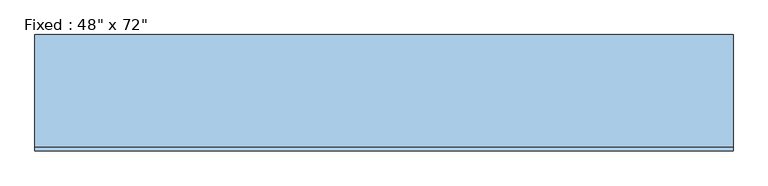
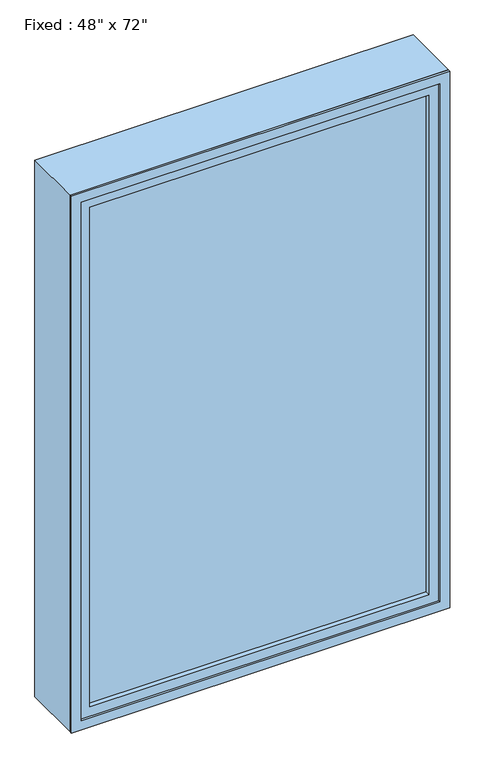
"""IFC4 building model written with IfcOpenShell, lengths in millimetres: window geometry."""

from ifc_helpers import new_model, si_unit, frame, origin, place, context, project, spatial, polyline, outline, extrude, source, transform, mapped, element, save


def window_b4876e44(model_context):
    return source(origin(), model_context, "Body", "SweptSolid", [
        extrude(outline(polyline([(508.0, -79.375), (-584.2, -79.375), (-584.2, -66.675), (508.0, -66.675), (508.0, -79.375)])), frame((0.0, 0.0, 368.3), z_axis=(0.0, 0.0, 1.0), x_axis=(1.0, 0.0, 0.0)), (0.0, 0.0, 1.0), 1701.8),
        extrude(outline(polyline([(2114.55, -628.65), (323.85, -628.65), (323.85, 552.45), (2114.55, 552.45), (2114.55, -628.65)]), holes=[polyline([(2070.1, -584.2), (2070.1, 508.0), (368.3, 508.0), (368.3, -584.2), (2070.1, -584.2)])]), frame((0.0, -95.25, 0.0), z_axis=(0.0, 1.0, 0.0), x_axis=(0.0, 0.0, 1.0)), (0.0, 0.0, 1.0), 44.45),
        extrude(outline(polyline([(2133.6, -647.7), (304.8, -647.7), (304.8, 571.5), (2133.6, 571.5), (2133.6, -647.7)]), holes=[polyline([(2101.85, -615.95), (2101.85, 539.75), (336.55, 539.75), (336.55, -615.95), (2101.85, -615.95)])]), frame((0.0, -101.6, 0.0), z_axis=(0.0, 1.0, 0.0), x_axis=(0.0, 0.0, 1.0)), (0.0, 0.0, 1.0), 6.35),
        extrude(outline(polyline([(2133.6, 571.5), (2133.6, -647.7), (304.8, -647.7), (304.8, 571.5), (2133.6, 571.5)]), holes=[polyline([(2114.55, 552.45), (323.85, 552.45), (323.85, -628.65), (2114.55, -628.65), (2114.55, 552.45)])]), frame((0.0, -95.25, 0.0), z_axis=(0.0, 1.0, 0.0), x_axis=(0.0, 0.0, 1.0)), (0.0, 0.0, 1.0), 196.85),
    ])


if __name__ == "__main__":
    model = new_model("IFC4")
    model_context = context("Model", 3, world=origin())
    ifc_project = project(units=[si_unit("LENGTHUNIT", "METRE", prefix="MILLI")], contexts=[model_context])
    site = spatial("IfcSite", under=ifc_project)
    building = spatial("IfcBuilding", under=site)
    placement = place(None, origin())
    window_shape = window_b4876e44(model_context)
    element("IfcWindow", 1, ObjectType="Fixed : 48\" x 72\"", at=placement, inside=building, context=model_context, shape_type="MappedRepresentation", body=[
        mapped(window_shape, transform((0.0, 0.0, 0.0), x_axis=(1.0, 0.0, 0.0), y_axis=(0.0, 1.0, 0.0), z_axis=(0.0, 0.0, 1.0))),
    ])
    save(model, "model.ifc")

# Revit data of these elements
# Type "Fixed : 48\" x 72\""
#   Type Mark = "13"
#   Construction Type Id = "GSP4R"
#   Assembly Code = "B2020100"
#   Analytic Construction = "1/8 in Pilkington single glazing"
#   Visual Light Transmittance = 0.9
#   Solar Heat Gain Coefficient = 0.78
#   Heat Transfer Coefficient (U) = 0.6496 BTU/(h·ft²·°F)
#   Height = 6' - 0"
#   Default Sill Height = 1' - 0"
#   Width = 4' - 0"
#   Window Inset = 0' - 6"
#   Define Thermal Properties by = 1
#   Glass Pane Material = Glass
#   Sash Material = Structure, Steel Bar Joist Layer
#   Wall Closure = (empty or 0)
# Element 1 (IfcWindow, "Fixed : 48\" x 72\"")
#   Materials on its faces: "Structure, Steel Bar Joist Layer", "Glass"
# Materials
#   "Glass": class "Glass", colour RGB 0 128 192, transparency 0.75, Description = "Soda Lime Glass", Cost = 0
#   "Structure, Steel Bar Joist Layer": class "Metal", colour RGB 127 127 127, transparency 0, Description = "Bar joists, thermal airspace", Cost = 0
